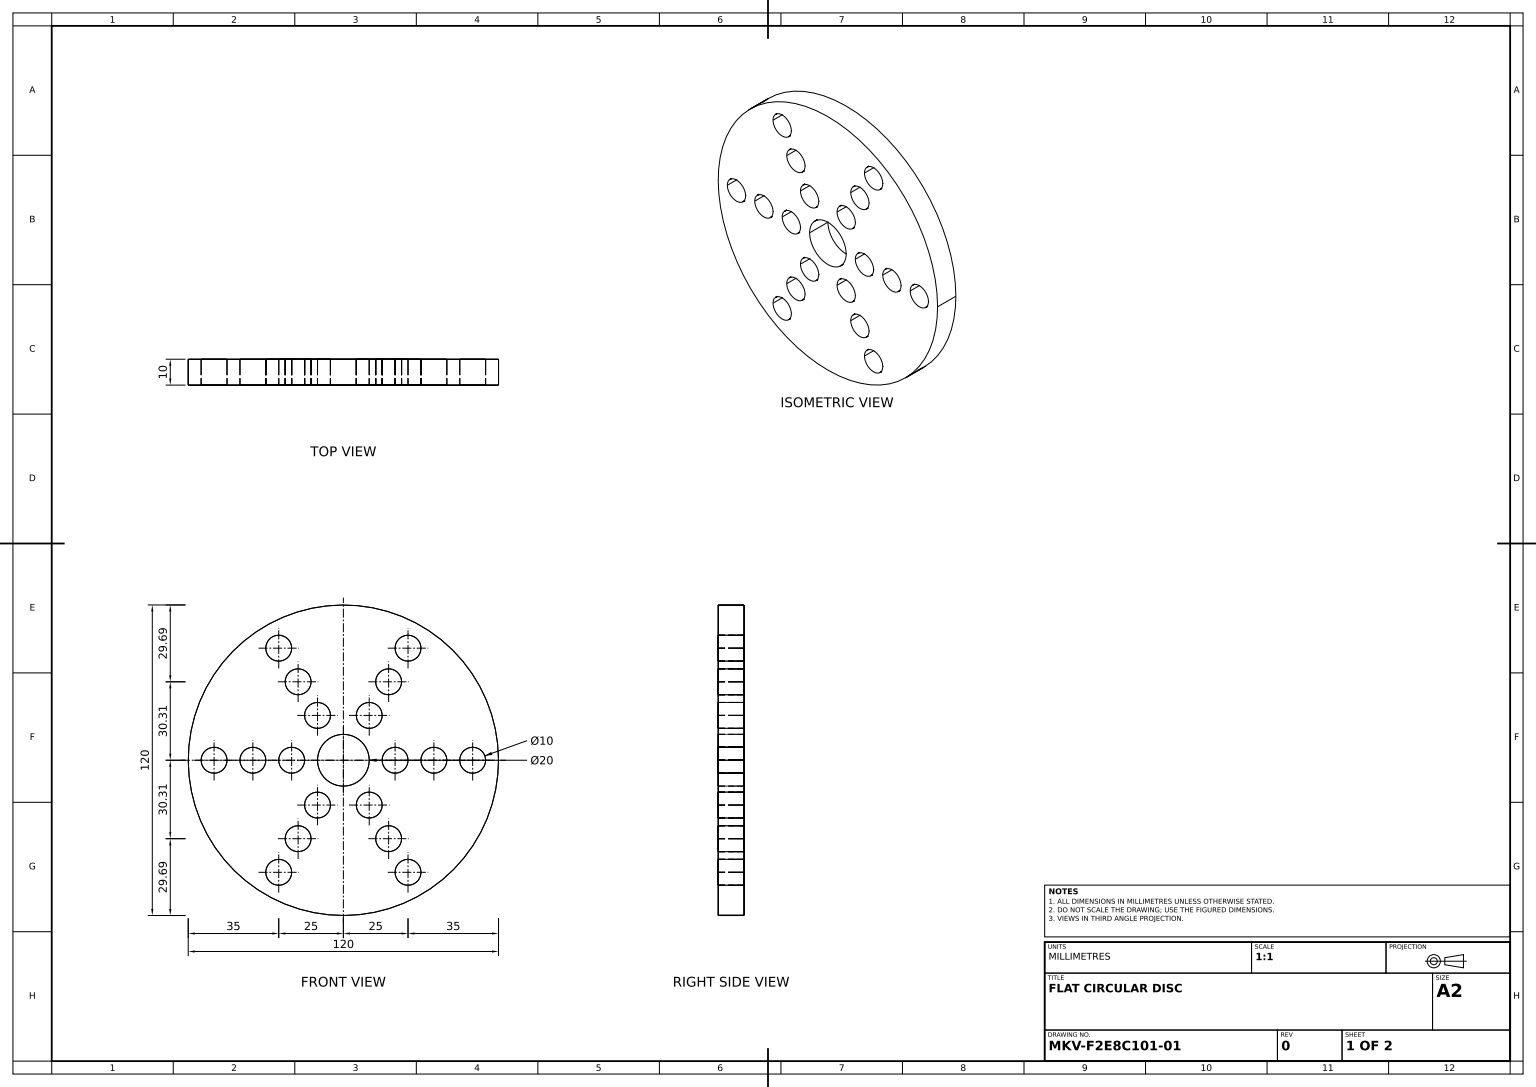
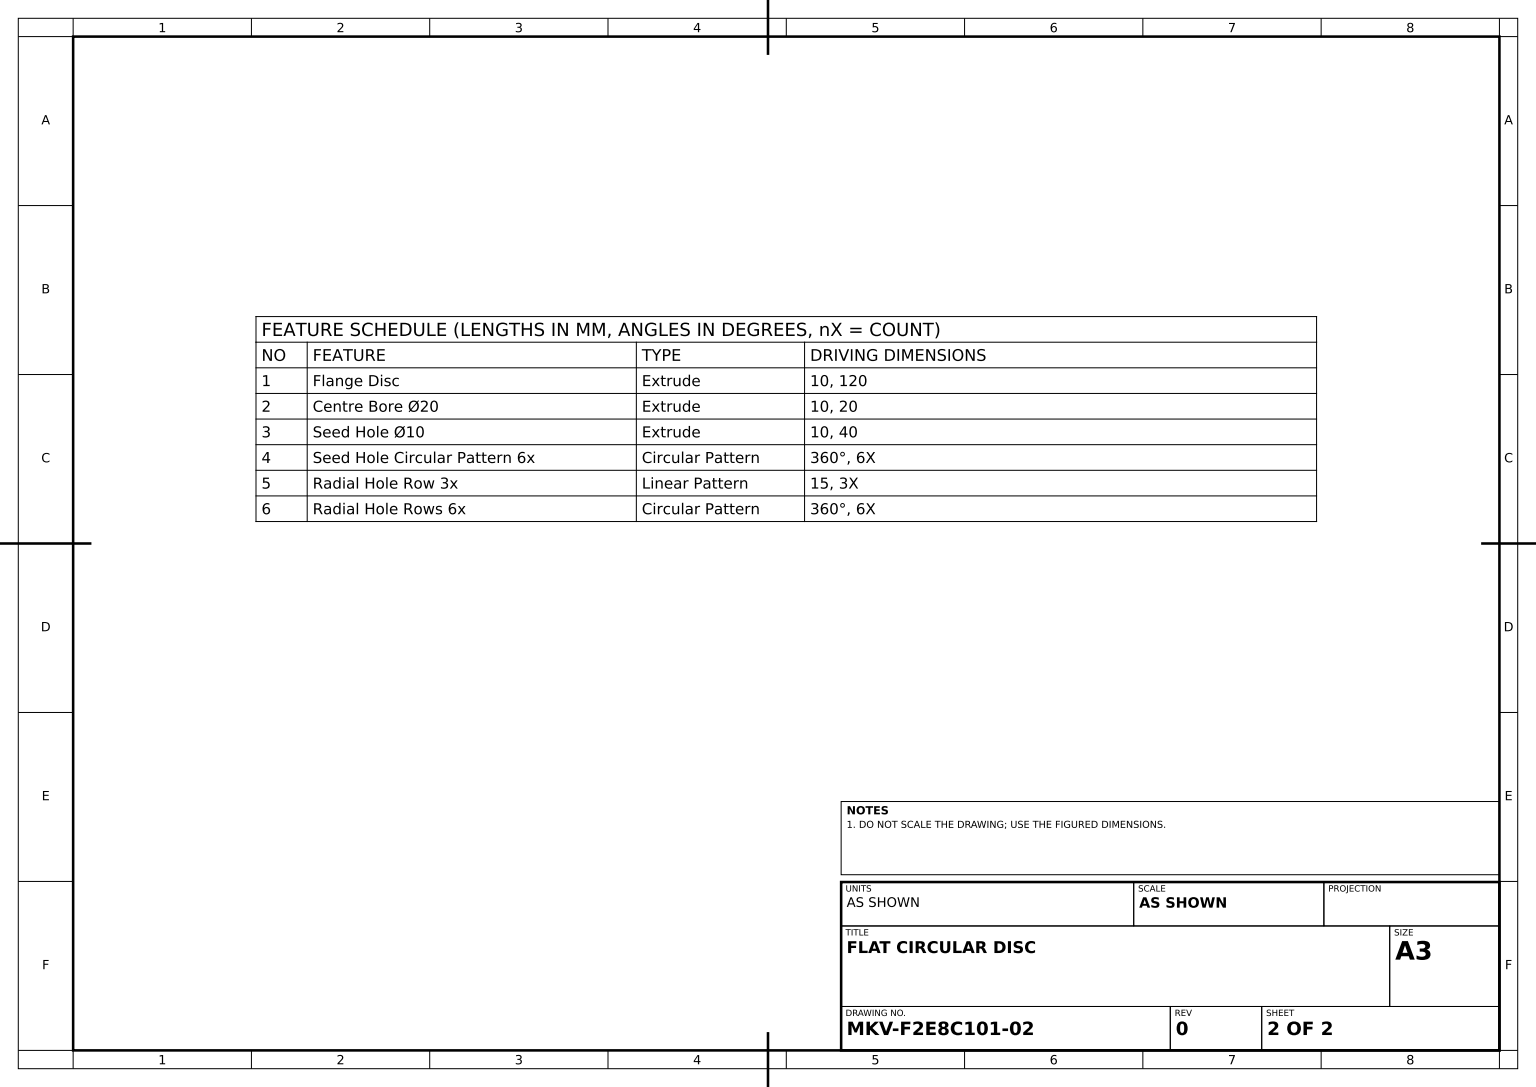
SolidWorks part; units mm, degrees
material "Plain Carbon Steel"
ref_plane "Front Plane" through (0, 0, 0) normal (0, 0, 1) x (1, 0, 0)
ref_plane "Top Plane" through (0, 0, 0) normal (0, 1, 0) x (1, 0, 0)
ref_plane "Right Plane" through (0, 0, 0) normal (1, 0, 0) x (0, 0, -1)
sketch "Flange Outline Ø120" plane through (0, 0, 0) normal (0, 0, 1) x (1, 0, 0)
  circle A0 centre (0, 0) radius 60
  dimension "D1" = 120
extrude "Flange Disc" add sketch "Flange Outline Ø120" along normal blind 10
sketch "Centre Bore Profile Ø20" plane through (0, 0, 10) normal (0, 0, 1) x (1, 0, 0)
  circle A0 centre (0, 0) radius 10
  dimension "D1" = 20
extrude "Centre Bore Ø20" cut sketch "Centre Bore Profile Ø20" against normal blind 10
sketch "Seed Hole Profile Ø10" plane through (0, 0, 10) normal (0, 0, 1) x (1, 0, 0)
  line L0 (0, 0) -> (20, 0) construction
  circle A0 centre (0, 0) radius 20 construction
  circle A1 centre (20, 0) radius 5
  dimension "D1" = 40
  dimension "D2" = 10
extrude "Seed Hole Ø10" cut sketch "Seed Hole Profile Ø10" against normal blind 10
pattern_circular "Seed Hole Circular Pattern 6x" count 6 over 360 about axis through (0, 0, 0) along (0, 0, 1) of "Seed Hole Ø10"
sketch "Radial Row Direction" plane through (0, 0, 10) normal (0, 0, 1) x (1, 0, 0)
  line L0 (0, 0) -> (60, 0) construction
  line L1 (0, 0) -> (-60, 0) construction
  circle A0 centre (0, 0) radius 60 construction
pattern_linear "Radial Hole Row 3x" count 3 spacing 15 along (1, 0, 0) of "Seed Hole Ø10"
pattern_circular "Radial Hole Rows 6x" count 6 over 360 about axis through (0, 0, 0) along (0, 0, 1) of "Radial Hole Row 3x"
